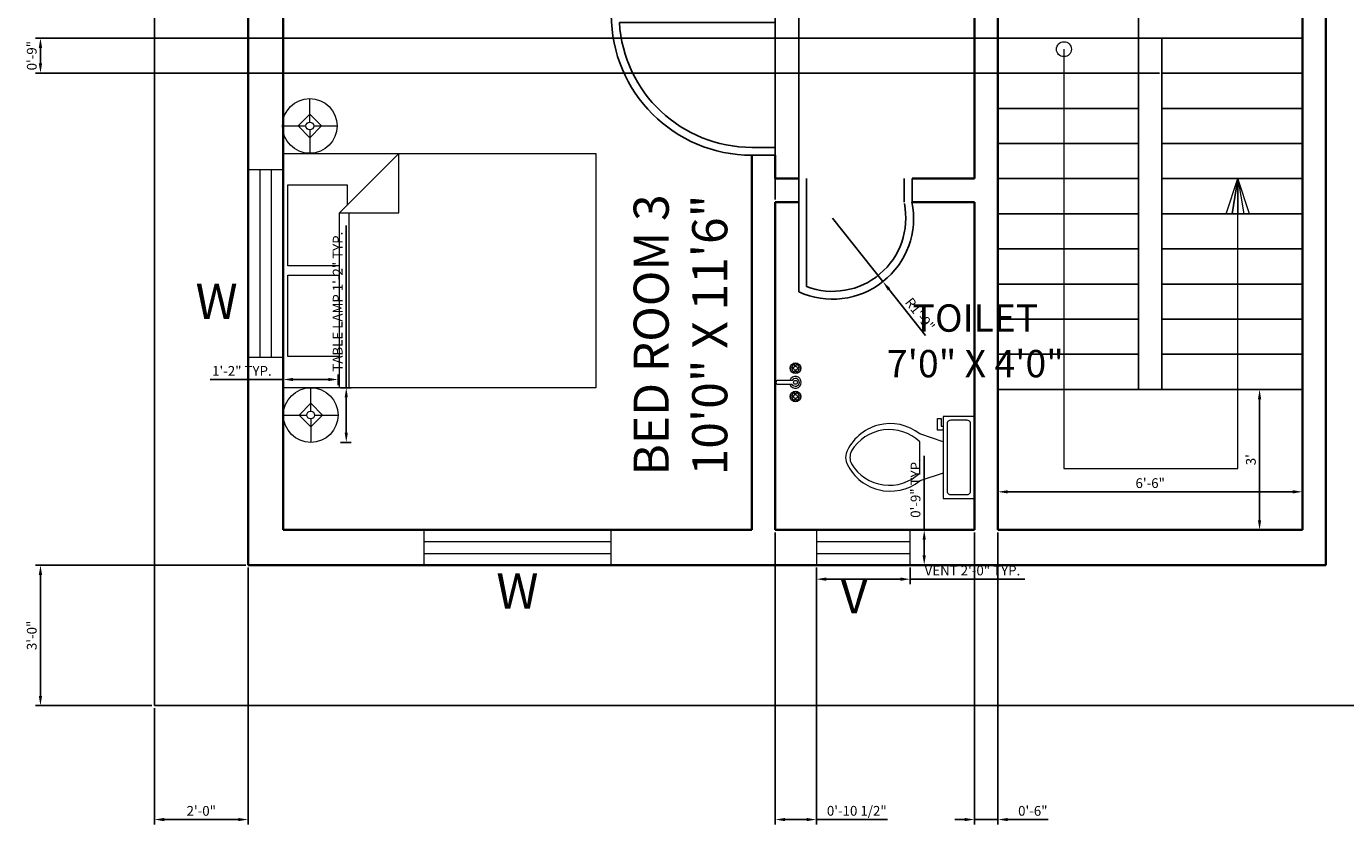
# Model space of a CAD drawing. Units: inches. Extents: x 1868 to 2413, y 1522 to 2138.
# Tile 1 of 4: x 1870 to 2207, y 1522 to 1727. Entities that reach past the tile are written whole.
import ezdxf

# ---------------------------------------------------------------- set-up
doc = ezdxf.new("R2010")
doc.units = ezdxf.units.IN
for name, color, linetype, lineweight in [('A-ANNO-DIMS', 2, 'Continuous', 18), ('A-ANNO-SYMB', 2, 'Continuous', 18), ('A-ANNO-TEXT', 7, 'Continuous', 18), ('A-AREA-IDEN', 7, 'Continuous', 25), ('A-DOOR', 3, 'Continuous', 25), ('A-FLOR-FIXT', 9, 'Continuous', 18), ('A-FLOR-STRS', 7, 'Continuous', 25), ('A-FURN', 8, 'Continuous', 18), ('A-GLAZ', 4, 'Continuous', 18), ('A-WALL', 7, 'Continuous', 35), ('C-PROP', 7, 'Continuous', 25)]:
    doc.layers.add(name, color=color, linetype=linetype, lineweight=lineweight)
doc.styles.get("Standard").update_dxf_attribs({"font": 'arial.ttf'})
doc.dimstyles.new('ISO-25', dxfattribs={"dimtxt": 2.5, "dimasz": 2.5, "dimexe": 1.25, "dimexo": 0.625, "dimtad": 1, "dimdec": 0, "dimlunit": 3, "dimtxsty": 'Standard', "dimcen": 2.5, "dimadec": 0, "dimazin": 0, "dimtfac": 1, "dimtdec": 0, "dimtmove": 0, "dimatfit": 3, "dimfxl": 1, "dimarcsym": 0})

# ---------------------------------------------------------------- blocks, each defined once
blk = doc.blocks.new('Faucet - Bathroom top')
for p, q in [((-4.107, 0.125), (-4.375, 0.125)), ((-3.75, 0.4788), (-3.75, 0.75)), ((-3.5, 0.482), (-3.5, 0.75)), ((-3.1461, 0.125), (-2.875, 0.125)), ((3.143, 0.125), (2.875, 0.125)), ((3.5, 0.4788), (3.5, 0.75)), ((3.75, 0.482), (3.75, 0.75)), ((4.1039, 0.125), (4.375, 0.125)), ((-4.1039, -0.125), (-4.375, -0.125)), ((-3.75, -0.4821), (-3.75, -0.75)), ((-3.5, -0.4789), (-3.5, -0.75)), ((-3.143, -0.125), (-2.875, -0.125)), ((-0.5, -0.8639), (-0.5, -4.5)), ((0.5, -4.5), (0.5, -0.8631)), ((3.1461, -0.125), (2.875, -0.125)), ((3.5, -0.4821), (3.5, -0.75)), ((3.75, -0.4789), (3.75, -0.75)), ((4.107, -0.125), (4.375, -0.125))]:
    blk.add_line(p, q)
for centre, radius in [((-3.625, 0), 1.375), ((-4.625, 0), 0.2795), ((-3.625, 0), 0.5), ((-3.625, 1), 0.2795), ((-2.625, 0), 0.2795), ((0, 0), 0.5), ((3.625, 0), 1.375), ((2.625, 0), 0.2795), ((3.625, 0), 0.5), ((3.625, 1), 0.2795), ((4.625, 0), 0.2795), ((-3.625, -1), 0.2795), ((3.625, -1), 0.2795)]:
    blk.add_circle(centre, radius)
for centre, radius, start, end in [((-3.625, 0), 1, 105.2407, 164.2093), ((-3.625, 0), 1, 16.44125, 74.07887), ((0, 0), 1.5, 289.6514, 250.3603), ((0, 0), 1, 300.3431, 239.7554), ((3.625, 0), 1, 106.12, 164.0884), ((3.625, 0), 1, 16.23422, 73.90469), ((-3.625, 0), 1, 196.2342, 253.9047), ((-3.625, 0), 1, 286.12, 344.0884), ((3.625, 0), 1, 196.4413, 254.0789), ((3.625, 0), 1, 285.2407, 344.2093), ((0, -4.5), 0.5, 180, 0)]:
    blk.add_arc(centre, radius, start, end)
blk = doc.blocks.new('Lamp - Table')
for p, q in [((0, 7), (0, 1)), ((-1, 0), (-7, 0)), ((0, 3), (-3, 0)), ((-3, 0), (0, -3)), ((3, 0), (0, 3)), ((0, -3), (3, 0)), ((1, 0), (7, 0)), ((0, -1), (0, -7))]:
    blk.add_line(p, q)
for radius in [7, 1]:
    blk.add_circle((0, 0), radius)
blk = doc.blocks.new('Bed - Queen')
for p, q in [((0, -80.00003), (0, 0)), ((0, 0), (59.99999, 0)), ((59.99999, 0), (59.99999, -80.00003)), ((7.99999, -1.2), (28.79998, -1.2)), ((7.99999, -14.4), (7.99999, -1.2)), ((28.79998, -1.2), (28.79998, -14.4)), ((31.19999, -1.2), (51.99999, -1.2)), ((31.19999, -14.4), (31.19999, -1.2)), ((51.99999, -1.2), (51.99999, -16.4)), ((0, -14.4), (44.8, -14.4)), ((44.8, -16.8), (0, -16.8)), ((59.99999, -29.6), (44.8, -14.4)), ((44.8, -14.4), (44.8, -29.6)), ((51.99999, -16.4), (46.79936, -16.4)), ((44.8, -29.6), (59.99999, -29.6)), ((59.99999, -80.00003), (0, -80.00003))]:
    blk.add_line(p, q)
blk = doc.blocks.new('Toilet - top')
for p, q in [((9.5, -6), (9.5, -2)), ((-10, -8.5), (-8, -8.5)), ((-10, -9.5), (-10, -8.5)), ((-7, -9.5), (-10, -9.5)), ((-8, -8.5), (-8, -8)), ((-7, -8), (-7, -9.5)), ((-4, -8), (-6, -14)), ((4, -8), (6, -14)), ((4, -14), (-4, -14))]:
    blk.add_line(p, q)
blk.add_lwpolyline([(10.5, -8), (10.5, 0), (-10.5, 0), (-10.5, -8)], close=True)
for points in [[(-9.5, -2), (-9.5, -6)], [(8.5, -1), (-8.5, -1)], [(-8.5, -7), (8.5, -7)]]:
    blk.add_lwpolyline(points)
for centre, radius, start, end in [((-8.62, -1.88), 0.884, 81.8699, 188.1301), ((8.62, -1.88), 0.884, 351.8699, 98.1301), ((-8.62, -6.12), 0.884, 171.8699, 278.1301), ((8.62, -6.12), 0.884, 261.8699, 8.1301), ((3.52, -21.58), 12.17, 141.4691, 247.9714), ((4.2, -21.82), 11.33, 136.3677, 238.9468), ((-3.52, -21.58), 12.17, 292.0284, 38.5307), ((-4.2, -21.82), 11.33, 301.053, 43.6321), ((0, -27.88), 4, 245.7318, 294.2682), ((0, -29), 4, 254.8605, 285.1395)]:
    blk.add_arc(centre, radius, start, end)
blk = doc.blocks.new('*D17')
at = {"layer": 'A-ANNO-DIMS', "color": 0, "lineweight": -2, "transparency": 16777216}
for p, q in [((2118.46, 1598.58), (2118.46, 1608.98)), ((2196.46, 1598.58), (2196.46, 1608.98)), ((2120.96, 1607.73), (2193.96, 1607.73))]:
    blk.add_line(p, q, dxfattribs=at)
at = {"layer": 'A-ANNO-DIMS', "color": 0, "transparency": 16777216}
for points in [[(2120.96, 1608.14), (2120.96, 1607.31), (2118.46, 1607.73)], [(2193.96, 1608.14), (2193.96, 1607.31), (2196.46, 1607.73)]]:
    blk.add_solid(points, dxfattribs=at)
at = {"layer": 'Defpoints', "color": 0, "transparency": 16777216}
for p in [(2196.46, 1607.73), (2118.46, 1597.95), (2196.46, 1597.95)]:
    blk.add_point(p, dxfattribs=at)
at = {"layer": 'A-ANNO-DIMS', "color": 0, "transparency": 16777216, "insert": (2157.46, 1609.63), "char_height": 2.5, "attachment_point": 5}
blk.add_mtext('6\'-6"', dxfattribs=at)
blk = doc.blocks.new('*D18')
at = {"layer": 'A-ANNO-DIMS', "color": 0, "lineweight": -2, "transparency": 16777216}
for p, q in [((2195.83, 1633.95), (2184.21, 1633.95)), ((2185.46, 1631.45), (2185.46, 1600.45)), ((2195.83, 1597.95), (2184.21, 1597.95))]:
    blk.add_line(p, q, dxfattribs=at)
at = {"layer": 'A-ANNO-DIMS', "color": 0, "transparency": 16777216}
for points in [[(2185.05, 1631.45), (2185.88, 1631.45), (2185.46, 1633.95)], [(2185.05, 1600.45), (2185.88, 1600.45), (2185.46, 1597.95)]]:
    blk.add_solid(points, dxfattribs=at)
at = {"layer": 'Defpoints', "color": 0, "transparency": 16777216}
for p in [(2196.46, 1633.95), (2185.46, 1597.95), (2196.46, 1597.95)]:
    blk.add_point(p, dxfattribs=at)
at = {"layer": 'A-ANNO-DIMS', "color": 0, "transparency": 16777216, "insert": (2183.56, 1615.95), "char_height": 2.5, "attachment_point": 5, "rotation": 90}
blk.add_mtext("3'", dxfattribs=at)
blk = doc.blocks.new('WIN-48IN')
for p, q in [((0, 48), (0, 0)), ((9, 48), (0, 48)), ((3, 48), (3, 0)), ((6, 0), (6, 48)), ((9, 0), (9, 48)), ((0, 0), (9, 0))]:
    blk.add_line(p, q)
blk = doc.blocks.new('VENT-24IN')
for p, q in [((24, 9), (0, 9)), ((0, 9), (0, 0)), ((24, 0), (24, 9)), ((24, 6), (0, 6)), ((0, 3), (24, 3)), ((0, 0), (24, 0))]:
    blk.add_line(p, q)
blk = doc.blocks.new('DOOR-36IN')
for p, q in [((36, 36), (0, 36)), ((0.06, 34), (0, 34)), ((36, 34), (2.06, 34)), ((36, 36), (42, 36)), ((36, 34), (42, 34)), ((42, 2), (36, 2)), ((42, 0), (36, 0))]:
    blk.add_line(p, q)
for radius, start in [(36, 180), (34, 183.3723)]:
    blk.add_arc((36, 36), radius, start, 270)
blk = doc.blocks.new('*D26')
at = {"layer": 'A-ANNO-DIMS', "color": 0, "lineweight": -2, "transparency": 16777216}
for p, q in [((2071.99, 1588.33), (2071.99, 1584.1)), ((2095.99, 1588.33), (2095.99, 1584.1)), ((2074.49, 1585.35), (2093.49, 1585.35)), ((2095.99, 1585.35), (2125.39, 1585.35))]:
    blk.add_line(p, q, dxfattribs=at)
at = {"layer": 'A-ANNO-DIMS', "color": 0, "transparency": 16777216}
for points in [[(2074.49, 1585.77), (2074.49, 1584.93), (2071.99, 1585.35)], [(2093.49, 1585.77), (2093.49, 1584.93), (2095.99, 1585.35)]]:
    blk.add_solid(points, dxfattribs=at)
at = {"layer": 'Defpoints', "color": 0, "transparency": 16777216}
for p in [(2071.99, 1588.95), (2095.99, 1588.95), (2095.99, 1585.35)]:
    blk.add_point(p, dxfattribs=at)
at = {"layer": 'A-ANNO-DIMS', "color": 0, "transparency": 16777216, "insert": (2111.94, 1587.25), "char_height": 2.5, "attachment_point": 5}
blk.add_mtext('VENT 2\'-0" TYP.', dxfattribs=at)
blk = doc.blocks.new('*D27')
at = {"layer": 'A-ANNO-DIMS', "color": 0, "lineweight": -2, "transparency": 16777216}
for p, q in [((2099.59, 1597.95), (2099.59, 1616.94)), ((2096.61, 1597.95), (2100.84, 1597.95)), ((2099.59, 1591.45), (2099.59, 1595.45)), ((2096.61, 1588.95), (2100.84, 1588.95))]:
    blk.add_line(p, q, dxfattribs=at)
at = {"layer": 'A-ANNO-DIMS', "color": 0, "transparency": 16777216}
for points in [[(2099.17, 1595.45), (2100, 1595.45), (2099.59, 1597.95)], [(2099.17, 1591.45), (2100, 1591.45), (2099.59, 1588.95)]]:
    blk.add_solid(points, dxfattribs=at)
at = {"layer": 'Defpoints', "color": 0, "transparency": 16777216}
for p in [(2095.99, 1597.95), (2099.59, 1597.95), (2095.99, 1588.95)]:
    blk.add_point(p, dxfattribs=at)
at = {"layer": 'A-ANNO-DIMS', "color": 0, "transparency": 16777216, "insert": (2097.69, 1608.7), "char_height": 2.5, "attachment_point": 5, "rotation": 90}
blk.add_mtext('0\'-9" TYP.', dxfattribs=at)
blk = doc.blocks.new('*D36')
at = {"layer": 'A-ANNO-DIMS', "color": 0, "lineweight": -2, "transparency": 16777216}
for p, q in [((1951.59, 1634.4), (1951.59, 1675.96)), ((1950.11, 1634.4), (1952.84, 1634.4)), ((1951.59, 1622.9), (1951.59, 1631.9)), ((1950.11, 1620.4), (1952.84, 1620.4))]:
    blk.add_line(p, q, dxfattribs=at)
at = {"layer": 'A-ANNO-DIMS', "color": 0, "transparency": 16777216}
for points in [[(1951.17, 1631.9), (1952, 1631.9), (1951.59, 1634.4)], [(1951.17, 1622.9), (1952, 1622.9), (1951.59, 1620.4)]]:
    blk.add_solid(points, dxfattribs=at)
at = {"layer": 'Defpoints', "color": 0, "transparency": 16777216}
for p in [(1949.49, 1634.4), (1951.59, 1634.4), (1949.49, 1620.4)]:
    blk.add_point(p, dxfattribs=at)
at = {"layer": 'A-ANNO-DIMS', "color": 0, "transparency": 16777216, "insert": (1949.71, 1656.43), "char_height": 2.5, "attachment_point": 5, "rotation": 90}
blk.add_mtext('TABLE LAMP 1\'-2" TYP.', dxfattribs=at)
blk = doc.blocks.new('*D37')
at = {"layer": 'A-ANNO-DIMS', "color": 0, "lineweight": -2, "transparency": 16777216}
for p, q in [((1935.49, 1636.5), (1916.73, 1636.5)), ((1935.49, 1635.02), (1935.49, 1637.75)), ((1946.99, 1636.5), (1937.99, 1636.5)), ((1949.49, 1635.02), (1949.49, 1637.75))]:
    blk.add_line(p, q, dxfattribs=at)
at = {"layer": 'A-ANNO-DIMS', "color": 0, "transparency": 16777216}
for points in [[(1937.99, 1636.91), (1937.99, 1636.08), (1935.49, 1636.5)], [(1946.99, 1636.91), (1946.99, 1636.08), (1949.49, 1636.5)]]:
    blk.add_solid(points, dxfattribs=at)
at = {"layer": 'Defpoints', "color": 0, "transparency": 16777216}
for p in [(1935.49, 1636.5), (1935.49, 1634.4), (1949.49, 1634.4)]:
    blk.add_point(p, dxfattribs=at)
at = {"layer": 'A-ANNO-DIMS', "color": 0, "transparency": 16777216, "insert": (1924.86, 1638.38), "char_height": 2.5, "attachment_point": 5}
blk.add_mtext('1\'-2" TYP.', dxfattribs=at)
blk = doc.blocks.new('*D52')
at = {"layer": 'A-ANNO-DIMS', "color": 0, "lineweight": -2, "transparency": 16777216}
for p, q in [((1926.46, 1588.33), (1926.46, 1522.53)), ((1902.46, 1552.33), (1902.46, 1522.53)), ((1904.96, 1523.78), (1923.96, 1523.78))]:
    blk.add_line(p, q, dxfattribs=at)
at = {"layer": 'A-ANNO-DIMS', "color": 0, "transparency": 16777216}
for points in [[(1904.96, 1524.19), (1904.96, 1523.36), (1902.46, 1523.78)], [(1923.96, 1524.19), (1923.96, 1523.36), (1926.46, 1523.78)]]:
    blk.add_solid(points, dxfattribs=at)
at = {"layer": 'Defpoints', "color": 0, "transparency": 16777216}
for p in [(1926.46, 1588.95), (1902.46, 1552.95), (1926.46, 1523.78)]:
    blk.add_point(p, dxfattribs=at)
at = {"layer": 'A-ANNO-DIMS', "color": 0, "transparency": 16777216, "insert": (1914.46, 1525.68), "char_height": 2.5, "attachment_point": 5}
blk.add_mtext('2\'-0"', dxfattribs=at)
blk = doc.blocks.new('*D53')
at = {"layer": 'A-ANNO-DIMS', "color": 0, "lineweight": -2, "transparency": 16777216}
for p, q in [((1925.83, 1588.95), (1872.03, 1588.95)), ((1873.28, 1555.45), (1873.28, 1586.45)), ((1901.83, 1552.95), (1872.03, 1552.95))]:
    blk.add_line(p, q, dxfattribs=at)
at = {"layer": 'A-ANNO-DIMS', "color": 0, "transparency": 16777216}
for points in [[(1872.86, 1586.45), (1873.7, 1586.45), (1873.28, 1588.95)], [(1872.86, 1555.45), (1873.7, 1555.45), (1873.28, 1552.95)]]:
    blk.add_solid(points, dxfattribs=at)
at = {"layer": 'Defpoints', "color": 0, "transparency": 16777216}
for p in [(1873.28, 1588.95), (1926.46, 1588.95), (1902.46, 1552.95)]:
    blk.add_point(p, dxfattribs=at)
at = {"layer": 'A-ANNO-DIMS', "color": 0, "transparency": 16777216, "insert": (1871.38, 1570.95), "char_height": 2.5, "attachment_point": 5, "rotation": 90}
blk.add_mtext('3\'-0"', dxfattribs=at)
blk = doc.blocks.new('*D54')
at = {"layer": 'A-ANNO-DIMS', "color": 0, "lineweight": -2, "transparency": 16777216}
for p, q in [((2118.46, 1706.58), (2118.46, 2135.38)), ((2154.46, 1706.58), (2154.46, 2135.38)), ((2120.96, 2134.13), (2151.96, 2134.13))]:
    blk.add_line(p, q, dxfattribs=at)
at = {"layer": 'A-ANNO-DIMS', "color": 0, "transparency": 16777216}
for points in [[(2120.96, 2134.54), (2120.96, 2133.71), (2118.46, 2134.13)], [(2151.96, 2134.54), (2151.96, 2133.71), (2154.46, 2134.13)]]:
    blk.add_solid(points, dxfattribs=at)
at = {"layer": 'Defpoints', "color": 0, "transparency": 16777216}
for p in [(2154.46, 2134.13), (2118.46, 1705.95), (2154.46, 1705.95)]:
    blk.add_point(p, dxfattribs=at)
at = {"layer": 'A-ANNO-DIMS', "color": 0, "transparency": 16777216, "insert": (2136.46, 2136.03), "char_height": 2.5, "attachment_point": 5}
blk.add_mtext('3\'-0"', dxfattribs=at)
blk = doc.blocks.new('*D55')
at = {"layer": 'A-ANNO-DIMS', "color": 0, "lineweight": -2, "transparency": 16777216}
for p, q in [((2159.83, 1723.95), (1872.03, 1723.95)), ((1873.28, 1721.45), (1873.28, 1717.45)), ((2159.83, 1714.95), (1872.03, 1714.95))]:
    blk.add_line(p, q, dxfattribs=at)
at = {"layer": 'A-ANNO-DIMS', "color": 0, "transparency": 16777216}
for points in [[(1872.86, 1721.45), (1873.7, 1721.45), (1873.28, 1723.95)], [(1872.86, 1717.45), (1873.7, 1717.45), (1873.28, 1714.95)]]:
    blk.add_solid(points, dxfattribs=at)
at = {"layer": 'Defpoints', "color": 0, "transparency": 16777216}
for p in [(2160.46, 1723.95), (1873.28, 1714.95), (2160.46, 1714.95)]:
    blk.add_point(p, dxfattribs=at)
at = {"layer": 'A-ANNO-DIMS', "color": 0, "transparency": 16777216, "insert": (1871.38, 1719.45), "char_height": 2.5, "attachment_point": 5, "rotation": 90}
blk.add_mtext('0\'-9"', dxfattribs=at)
blk = doc.blocks.new('*D60')
at = {"layer": 'A-ANNO-DIMS', "color": 0, "lineweight": -2, "transparency": 16777216}
for p, q in [((2061.46, 1597.33), (2061.46, 1522.53)), ((2071.99, 1588.33), (2071.99, 1522.53)), ((2063.96, 1523.78), (2069.49, 1523.78)), ((2071.99, 1523.78), (2090.15, 1523.78))]:
    blk.add_line(p, q, dxfattribs=at)
at = {"layer": 'A-ANNO-DIMS', "color": 0, "transparency": 16777216}
for points in [[(2063.96, 1524.19), (2063.96, 1523.36), (2061.46, 1523.78)], [(2069.49, 1524.19), (2069.49, 1523.36), (2071.99, 1523.78)]]:
    blk.add_solid(points, dxfattribs=at)
at = {"layer": 'Defpoints', "color": 0, "transparency": 16777216}
for p in [(2061.46, 1597.95), (2071.99, 1588.95), (2071.99, 1523.78)]:
    blk.add_point(p, dxfattribs=at)
at = {"layer": 'A-ANNO-DIMS', "color": 0, "transparency": 16777216, "insert": (2082.32, 1525.69), "char_height": 2.5, "attachment_point": 5}
blk.add_mtext('0\'-10 1/2"', dxfattribs=at)
blk = doc.blocks.new('*D61')
at = {"layer": 'A-ANNO-DIMS', "color": 0, "lineweight": -2, "transparency": 16777216}
for p, q in [((2061.46, 1682.58), (2061.46, 2135.38)), ((2067.46, 1682.58), (2067.46, 2135.38)), ((2058.96, 2134.13), (2056.46, 2134.13)), ((2061.46, 2134.13), (2067.46, 2134.13)), ((2069.96, 2134.13), (2080.35, 2134.13))]:
    blk.add_line(p, q, dxfattribs=at)
at = {"layer": 'A-ANNO-DIMS', "color": 0, "transparency": 16777216}
for points in [[(2058.96, 2134.54), (2058.96, 2133.71), (2061.46, 2134.13)], [(2069.96, 2134.54), (2069.96, 2133.71), (2067.46, 2134.13)]]:
    blk.add_solid(points, dxfattribs=at)
at = {"layer": 'Defpoints', "color": 0, "transparency": 16777216}
for p in [(2067.46, 2134.13), (2061.46, 1681.95), (2067.46, 1681.95)]:
    blk.add_point(p, dxfattribs=at)
at = {"layer": 'A-ANNO-DIMS', "color": 0, "transparency": 16777216, "insert": (2076.4, 2136.03), "char_height": 2.5, "attachment_point": 5}
blk.add_mtext('0\'-6"', dxfattribs=at)
blk = doc.blocks.new('*D64')
at = {"layer": 'A-ANNO-DIMS', "color": 0, "lineweight": -2, "transparency": 16777216}
for p, q in [((2112.46, 1597.33), (2112.46, 1522.53)), ((2118.46, 1597.33), (2118.46, 1522.53)), ((2109.96, 1523.78), (2107.46, 1523.78)), ((2112.46, 1523.78), (2118.46, 1523.78)), ((2120.96, 1523.78), (2131.35, 1523.78))]:
    blk.add_line(p, q, dxfattribs=at)
at = {"layer": 'A-ANNO-DIMS', "color": 0, "transparency": 16777216}
for points in [[(2109.96, 1524.19), (2109.96, 1523.36), (2112.46, 1523.78)], [(2120.96, 1524.19), (2120.96, 1523.36), (2118.46, 1523.78)]]:
    blk.add_solid(points, dxfattribs=at)
at = {"layer": 'Defpoints', "color": 0, "transparency": 16777216}
for p in [(2112.46, 1597.95), (2118.46, 1597.95), (2118.46, 1523.78)]:
    blk.add_point(p, dxfattribs=at)
at = {"layer": 'A-ANNO-DIMS', "color": 0, "transparency": 16777216, "insert": (2127.4, 1525.68), "char_height": 2.5, "attachment_point": 5}
blk.add_mtext('0\'-6"', dxfattribs=at)
blk = doc.blocks.new('*D65')
at = {"layer": 'A-ANNO-DIMS', "color": 0, "lineweight": -2, "transparency": 16777216}
for p, q in [((2076.11, 1677.83), (2089.01, 1661.56)), ((2099.95, 1647.77), (2090.56, 1659.6))]:
    blk.add_line(p, q, dxfattribs=at)
at = {"layer": 'A-ANNO-DIMS', "color": 0, "transparency": 16777216}
blk.add_solid([(2090.89, 1659.86), (2090.24, 1659.34), (2089.01, 1661.56)], dxfattribs=at)
at = {"layer": 'Defpoints', "color": 0, "transparency": 16777216}
for p in [(2076.11, 1677.83), (2089.01, 1661.56)]:
    blk.add_point(p, dxfattribs=at)
at = {"layer": 'A-ANNO-DIMS', "color": 0, "transparency": 16777216, "insert": (2098.24, 1652.98), "char_height": 2.5, "attachment_point": 5, "rotation": 308.4179}
blk.add_mtext('R1\'-9"', dxfattribs=at)

msp = doc.modelspace()

# ---------------------------------------------------------------- linework, layer by layer
at = {"layer": 'A-ANNO-SYMB'}
for p, q in [((2135.36, 1721.11), (2135.36, 1613.72)), ((2176.91, 1678.95), (2179.91, 1687.95)), ((2179.91, 1687.95), (2178.41, 1678.95)), ((2178.41, 1678.95), (2179.91, 1687.95)), ((2179.91, 1687.95), (2179.91, 1687.95)), ((2182.91, 1678.95), (2179.91, 1687.95)), ((2179.91, 1687.95), (2179.91, 1678.95)), ((2179.91, 1678.95), (2179.91, 1687.95)), ((2179.91, 1687.95), (2181.41, 1678.95)), ((2179.91, 1678.95), (2176.91, 1678.95)), ((2179.91, 1613.72), (2179.91, 1678.95)), ((2179.91, 1678.95), (2182.91, 1678.95)), ((2135.36, 1613.72), (2179.91, 1613.72))]:
    msp.add_line(p, q, dxfattribs=at)
msp.add_circle((2135.36, 1721.11), 1.91, dxfattribs=at)
at = {"layer": 'A-DOOR'}
for p, q in [((2067.46, 1687.95), (2067.46, 1681.95)), ((2067.46, 1687.95), (2067.46, 1658.95)), ((2069.46, 1687.95), (2069.46, 1660.28)), ((2094.46, 1681.95), (2094.46, 1687.95)), ((2096.46, 1681.95), (2096.46, 1687.95))]:
    msp.add_line(p, q, dxfattribs=at)
for radius, start in [(20.76, 245.3845), (18.76, 249.2471)]:
    msp.add_arc((2076.11, 1677.83), radius, start, 11.4516, dxfattribs=at)
at = {"layer": 'A-FLOR-STRS'}
for p, q in [((2154.46, 1633.95), (2154.46, 1723.95)), ((2154.46, 1723.95), (2196.46, 1723.95)), ((2160.46, 1633.95), (2160.46, 1723.95)), ((2160.46, 1714.95), (2196.46, 1714.95)), ((2118.46, 1705.95), (2154.46, 1705.95)), ((2160.46, 1705.95), (2196.46, 1705.95)), ((2118.46, 1696.95), (2154.46, 1696.95)), ((2160.46, 1696.95), (2196.46, 1696.95)), ((2118.46, 1687.95), (2154.46, 1687.95)), ((2160.46, 1687.95), (2196.46, 1687.95)), ((2118.46, 1678.95), (2154.46, 1678.95)), ((2160.46, 1678.95), (2196.46, 1678.95)), ((2118.46, 1669.95), (2154.46, 1669.95)), ((2160.46, 1669.95), (2196.46, 1669.95)), ((2118.46, 1660.95), (2154.46, 1660.95)), ((2160.46, 1660.95), (2196.46, 1660.95)), ((2118.46, 1651.95), (2154.46, 1651.95)), ((2160.46, 1651.95), (2196.46, 1651.95)), ((2118.46, 1642.95), (2154.46, 1642.95)), ((2160.46, 1642.95), (2196.46, 1642.95)), ((2118.46, 1633.95), (2196.46, 1633.95))]:
    msp.add_line(p, q, dxfattribs=at)
at = {"layer": 'A-WALL'}
for p, q in [((1926.46, 2078.95), (1926.46, 1588.95)), ((1935.46, 1919.95), (1935.46, 1597.95)), ((2112.46, 1687.95), (2112.46, 1747.95)), ((2118.46, 1597.95), (2118.46, 1747.95)), ((2196.46, 1597.95), (2196.46, 1747.95)), ((2202.46, 1597.95), (2202.46, 1747.95)), ((2055.46, 1693.95), (2055.46, 1597.95)), ((2061.46, 1693.95), (2061.46, 1687.95)), ((2061.46, 1687.95), (2067.46, 1687.95)), ((2061.46, 1687.95), (2067.46, 1687.95)), ((2096.46, 1687.95), (2112.46, 1687.95)), ((2061.46, 1681.95), (2067.46, 1681.95)), ((2061.46, 1681.95), (2061.46, 1597.95)), ((2096.46, 1681.95), (2112.46, 1681.95)), ((2112.46, 1597.95), (2112.46, 1681.95)), ((1935.46, 1597.95), (2055.46, 1597.95)), ((2061.46, 1597.95), (2112.46, 1597.95)), ((2118.46, 1597.95), (2196.46, 1597.95)), ((2202.46, 1597.95), (2202.46, 1588.95)), ((1926.46, 1588.95), (2202.46, 1588.95))]:
    msp.add_line(p, q, dxfattribs=at)
at = {"layer": 'C-PROP'}
for p, q in [((1902.46, 2104.95), (1902.46, 1552.95)), ((1902.46, 1552.95), (2382.46, 1552.95))]:
    msp.add_line(p, q, dxfattribs=at)

# ---------------------------------------------------------------- block references
at = {"layer": 'A-DOOR'}
msp.add_blockref('DOOR-36IN', (2019.46, 1693.95), dxfattribs=at)
at = {"layer": 'A-FLOR-FIXT', "rotation": 270}
for name, p in [('Faucet - Bathroom top', (2066.62, 1635.76)), ('Toilet - top', (2112.46, 1616.54))]:
    msp.add_blockref(name, p, dxfattribs=at)
at = {"layer": 'A-FURN', "rotation": 90}
for name, p in [('Lamp - Table', (1942.25, 1701.44)), ('Bed - Queen', (1935.46, 1634.39)), ('Lamp - Table', (1942.49, 1627.4))]:
    msp.add_blockref(name, p, dxfattribs=at)
at = {"layer": 'A-GLAZ'}
for name, p in [('WIN-48IN', (1926.46, 1642.2)), ('VENT-24IN', (2071.99, 1588.95))]:
    msp.add_blockref(name, p, dxfattribs=at)
at = {"layer": 'A-GLAZ', "rotation": 270.0000000000012}
msp.add_blockref('WIN-48IN', (1971.46, 1597.95), dxfattribs=at)

# ---------------------------------------------------------------- texts
at = {"layer": 'A-ANNO-TEXT', "char_height": 9, "attachment_point": 1}
for s, insert in [('\\pxqc;W', (1876.49, 1661.03)), ('\\pxqc;W', (1953.52, 1586.82)), ('\\pxqc;V', (2039.74, 1585.6))]:
    msp.add_mtext_dynamic_manual_height_columns(s, width=83.7859, gutter_width=12.5, heights=[0], dxfattribs=dict(at, insert=insert))
at = {"layer": 'A-AREA-IDEN', "insert": (2025.17, 1584.34), "char_height": 9, "attachment_point": 1, "rotation": 90}
msp.add_mtext_dynamic_manual_height_columns('\\pxqc;BED ROOM 3\\P10\'0" X 11\'6"', width=127.1139, gutter_width=12.5, heights=[0], dxfattribs=at)
at = {"layer": 'A-AREA-IDEN', "insert": (2089.81, 1655.73), "char_height": 7, "attachment_point": 1}
msp.add_mtext('\\pxqc;TOILET\\P7\'0" X 4\'0"', dxfattribs=at)

# ---------------------------------------------------------------- dimensions: what is measured, and where the dimension line sits
at = {"layer": 'A-ANNO-DIMS'}
for base, p1, p2, override, picture, middle in [((2067.46, 2134.13), (2061.46, 1681.95), (2067.46, 1681.95), {"dimdec": 1, "dimlfac": 1, "dimrnd": 0, "dimzin": 1, "dimdsep": 46, "dimlunit": 4, "dimfrac": 2}, '*D61', (2076.4, 2136.03)), ((2154.46, 2134.13), (2118.46, 1705.95), (2154.46, 1705.95), {"dimdec": 1, "dimlfac": 1, "dimrnd": 0, "dimzin": 1, "dimdsep": 46, "dimlunit": 4, "dimfrac": 2}, '*D54', (2136.46, 2136.03)), ((2196.46, 1607.73), (2118.46, 1597.95), (2196.46, 1597.95), {"dimclrd": 0, "dimclre": 0, "dimclrt": 0}, '*D17', (2157.46, 1609.63)), ((2071.99, 1523.78), (2061.46, 1597.95), (2071.99, 1588.95), {"dimdec": 1, "dimlfac": 1, "dimrnd": 0, "dimzin": 1, "dimdsep": 46, "dimlunit": 4, "dimfrac": 2}, '*D60', (2082.32, 1525.69)), ((2118.46, 1523.78), (2112.46, 1597.95), (2118.46, 1597.95), {"dimdec": 1, "dimlfac": 1, "dimrnd": 0, "dimzin": 1, "dimdsep": 46, "dimlunit": 4, "dimfrac": 2}, '*D64', (2127.4, 1525.68)), ((1926.46, 1523.78), (1902.46, 1552.95), (1926.46, 1588.95), {"dimdec": 1, "dimlfac": 1, "dimrnd": 0, "dimzin": 1, "dimdsep": 46, "dimlunit": 4, "dimfrac": 2}, '*D52', (1914.46, 1525.68))]:
    dim = msp.add_linear_dim(base=base, p1=p1, p2=p2, dimstyle='ISO-25', override=override, dxfattribs=at)
    dim.commit()
    dim.dimension.update_dxf_attribs({"geometry": picture, "text_midpoint": middle})
for base, p1, p2, override, picture, middle in [((1873.28, 1714.95), (2160.46, 1723.95), (2160.46, 1714.95), {"dimdec": 1, "dimlfac": 1, "dimrnd": 0, "dimzin": 1, "dimdsep": 46, "dimlunit": 4, "dimfrac": 2}, '*D55', (1871.38, 1719.45)), ((2185.46, 1597.95), (2196.46, 1633.95), (2196.46, 1597.95), {"dimclrd": 0, "dimclre": 0, "dimclrt": 0}, '*D18', (2183.56, 1615.95)), ((1873.28, 1588.95), (1902.46, 1552.95), (1926.46, 1588.95), {"dimdec": 1, "dimlfac": 1, "dimrnd": 0, "dimzin": 1, "dimdsep": 46, "dimlunit": 4, "dimfrac": 2}, '*D53', (1871.38, 1570.95))]:
    dim = msp.add_linear_dim(base=base, p1=p1, p2=p2, angle=90, dimstyle='ISO-25', override=override, dxfattribs=at)
    dim.commit()
    dim.dimension.update_dxf_attribs({"geometry": picture, "text_midpoint": middle})
for base, p1, p2, angle, text, picture, middle in [((1951.59, 1634.4), (1949.49, 1620.4), (1949.49, 1634.4), 90, 'TABLE LAMP <> TYP.', '*D36', (1949.71, 1656.43)), ((1935.49, 1636.5), (1949.49, 1634.4), (1935.49, 1634.4), 180, '<> TYP.', '*D37', (1924.86, 1638.38)), ((2099.59, 1597.95), (2095.99, 1588.95), (2095.99, 1597.95), 90, '<> TYP.', '*D27', (2097.69, 1608.7))]:
    dim = msp.add_linear_dim(base=base, p1=p1, p2=p2, angle=angle, text=text, dimstyle='ISO-25', override={"dimdec": 1, "dimlfac": 1, "dimrnd": 0, "dimzin": 1, "dimdsep": 46, "dimlunit": 4, "dimfrac": 2}, dxfattribs=at)
    dim.commit()
    dim.dimension.update_dxf_attribs({"geometry": picture, "text_midpoint": middle})
dim = msp.add_radius_dim(center=(2076.11, 1677.83), mpoint=(2089.01, 1661.56), dimstyle='ISO-25', override={"dimdec": 1, "dimlfac": 1, "dimrnd": 0, "dimzin": 1, "dimdsep": 46, "dimlunit": 4, "dimfrac": 2}, dxfattribs=at)
dim.commit()
dim.dimension.update_dxf_attribs({"geometry": '*D65', "text_midpoint": (2096.75, 1651.8), "dimtype": 164})
dim = msp.add_linear_dim(base=(2095.99, 1585.35), p1=(2071.99, 1588.95), p2=(2095.99, 1588.95), text='VENT <> TYP.', dimstyle='ISO-25', override={"dimdec": 1, "dimlfac": 1, "dimrnd": 0, "dimzin": 1, "dimdsep": 46, "dimlunit": 4, "dimfrac": 2}, dxfattribs=at)
dim.commit()
dim.dimension.update_dxf_attribs({"geometry": '*D26', "text_midpoint": (2111.94, 1587.25)})

doc.saveas('drawing.dxf')
